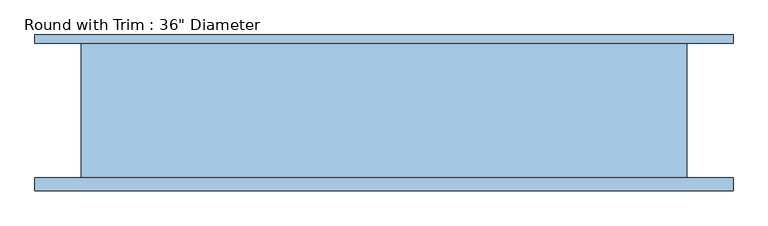
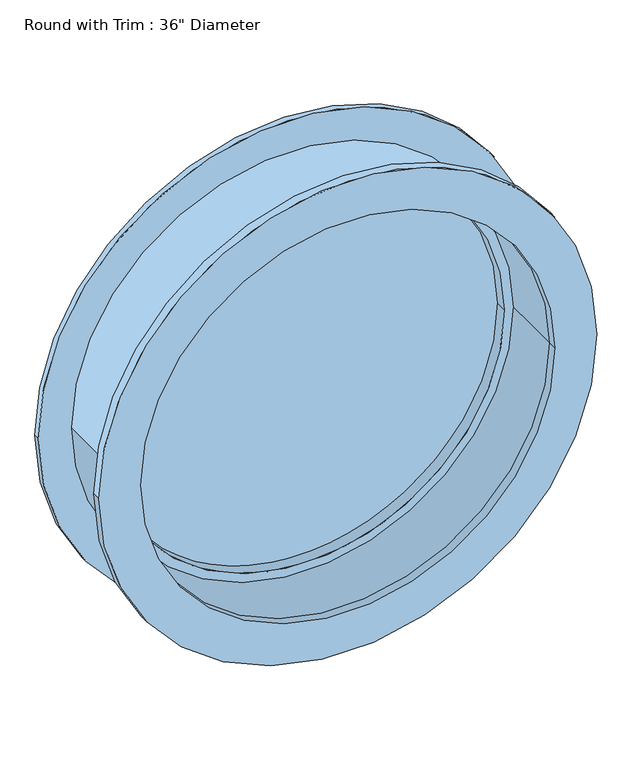
"""IFC4 building model written with IfcOpenShell, lengths in millimetres: window geometry."""

from ifc_helpers import new_model, si_unit, point, frame, frame_2d, origin, place, context, project, spatial, circle_curve, trimmed, segment, composite_curve, outline, extrude, source, transform, mapped, element, save


def window_736d8d37(model_context):
    return source(origin(), model_context, "Body", "SweptSolid", [
        extrude(outline(composite_curve([segment(trimmed(circle_curve(frame_2d((1219.2, 0.0)), 527.05), [point((1219.2, -527.05))], [point((1219.2, 527.05))], False, "CARTESIAN"), True, "CONTINUOUS"), segment(trimmed(circle_curve(frame_2d((1219.2, 0.0)), 527.05), [point((1219.2, 527.05))], [point((1219.2, -527.05))], False, "CARTESIAN"), True, "CONTINUOUS")], self_intersect=False), holes=[composite_curve([segment(trimmed(circle_curve(frame_2d((1219.2, 0.0)), 438.15), [point((1219.2, -438.15))], [point((1219.2, 438.15))], True, "CARTESIAN"), True, "CONTINUOUS"), segment(trimmed(circle_curve(frame_2d((1219.2, 0.0)), 438.15), [point((1219.2, 438.15))], [point((1219.2, -438.15))], True, "CARTESIAN"), True, "CONTINUOUS")], self_intersect=False)]), frame((0.0, -120.65, 0.0), z_axis=(0.0, 1.0, 0.0), x_axis=(0.0, 0.0, 1.0)), (0.0, 0.0, 1.0), 19.05),
        extrude(outline(composite_curve([segment(trimmed(circle_curve(frame_2d((1219.2, 0.0)), 527.05), [point((1219.2, -527.05))], [point((1219.2, 527.05))], False, "CARTESIAN"), True, "CONTINUOUS"), segment(trimmed(circle_curve(frame_2d((1219.2, 0.0)), 527.05), [point((1219.2, 527.05))], [point((1219.2, -527.05))], False, "CARTESIAN"), True, "CONTINUOUS")], self_intersect=False), holes=[composite_curve([segment(trimmed(circle_curve(frame_2d((1219.2, 0.0)), 438.15), [point((1219.2, -438.15))], [point((1219.2, 438.15))], True, "CARTESIAN"), True, "CONTINUOUS"), segment(trimmed(circle_curve(frame_2d((1219.2, 0.0)), 438.15), [point((1219.2, 438.15))], [point((1219.2, -438.15))], True, "CARTESIAN"), True, "CONTINUOUS")], self_intersect=False)]), frame((0.0, 101.6, 0.0), z_axis=(0.0, 1.0, 0.0), x_axis=(0.0, 0.0, 1.0)), (0.0, 0.0, 1.0), 12.7),
        extrude(outline(composite_curve([segment(trimmed(circle_curve(frame_2d((1219.2, 0.0)), 419.1), [point((1219.2, -419.1))], [point((1219.2, 419.1))], False, "CARTESIAN"), True, "CONTINUOUS"), segment(trimmed(circle_curve(frame_2d((1219.2, 0.0)), 419.1), [point((1219.2, 419.1))], [point((1219.2, -419.1))], False, "CARTESIAN"), True, "CONTINUOUS")], self_intersect=False)), frame((0.0, 57.15, 0.0), z_axis=(0.0, 1.0, 0.0), x_axis=(0.0, 0.0, 1.0)), (0.0, 0.0, 1.0), 12.7),
        extrude(outline(composite_curve([segment(trimmed(circle_curve(frame_2d((1219.2, 0.0)), 438.15), [point((1219.2, -438.15))], [point((1219.2, 438.15))], False, "CARTESIAN"), True, "CONTINUOUS"), segment(trimmed(circle_curve(frame_2d((1219.2, 0.0)), 438.15), [point((1219.2, 438.15))], [point((1219.2, -438.15))], False, "CARTESIAN"), True, "CONTINUOUS")], self_intersect=False), holes=[composite_curve([segment(trimmed(circle_curve(frame_2d((1219.2, 0.0)), 419.1), [point((1219.2, -419.1))], [point((1219.2, 419.1))], True, "CARTESIAN"), True, "CONTINUOUS"), segment(trimmed(circle_curve(frame_2d((1219.2, 0.0)), 419.1), [point((1219.2, 419.1))], [point((1219.2, -419.1))], True, "CARTESIAN"), True, "CONTINUOUS")], self_intersect=False)]), frame((0.0, 31.75, 0.0), z_axis=(0.0, 1.0, 0.0), x_axis=(0.0, 0.0, 1.0)), (0.0, 0.0, 1.0), 50.8),
        extrude(outline(composite_curve([segment(trimmed(circle_curve(frame_2d((1219.2, 0.0)), 457.2), [point((1219.2, -457.2))], [point((1219.2, 457.2))], False, "CARTESIAN"), True, "CONTINUOUS"), segment(trimmed(circle_curve(frame_2d((1219.2, 0.0)), 457.2), [point((1219.2, 457.2))], [point((1219.2, -457.2))], False, "CARTESIAN"), True, "CONTINUOUS")], self_intersect=False), holes=[composite_curve([segment(trimmed(circle_curve(frame_2d((1219.2, 0.0)), 438.15), [point((1219.2, -438.15))], [point((1219.2, 438.15))], True, "CARTESIAN"), True, "CONTINUOUS"), segment(trimmed(circle_curve(frame_2d((1219.2, 0.0)), 438.15), [point((1219.2, 438.15))], [point((1219.2, -438.15))], True, "CARTESIAN"), True, "CONTINUOUS")], self_intersect=False)]), frame((0.0, -101.6, 0.0), z_axis=(0.0, 1.0, 0.0), x_axis=(0.0, 0.0, 1.0)), (0.0, 0.0, 1.0), 203.2),
    ])


if __name__ == "__main__":
    model = new_model("IFC4")
    model_context = context("Model", 3, world=origin())
    ifc_project = project(units=[si_unit("LENGTHUNIT", "METRE", prefix="MILLI")], contexts=[model_context])
    site = spatial("IfcSite", under=ifc_project)
    building = spatial("IfcBuilding", under=site)
    placement = place(None, origin())
    window_shape = window_736d8d37(model_context)
    element("IfcWindow", 1, ObjectType="Round with Trim : 36\" Diameter", at=placement, inside=building, context=model_context, shape_type="MappedRepresentation", body=[
        mapped(window_shape, transform((0.0, 0.0, 0.0), x_axis=(1.0, 0.0, 0.0), y_axis=(0.0, 1.0, 0.0), z_axis=(0.0, 0.0, 1.0))),
    ])
    save(model, "model.ifc")

# Revit data of these elements
# Type "Round with Trim : 36\" Diameter"
#   Type Mark = "24"
#   Construction Type Id = "GSP4R"
#   Assembly Code = "B2020100"
#   Analytic Construction = "1/8 in Pilkington single glazing"
#   Visual Light Transmittance = 0.9
#   Solar Heat Gain Coefficient = 0.78
#   Heat Transfer Coefficient (U) = 0.6496 BTU/(h·ft²·°F)
#   Default Sill Height = 2' - 6"
#   Trim Projection - Ext. = 0' - 0 1/2"
#   Trim Projection - Int. = 0' - 0 3/4"
#   Trim Width - Exterior = 0' - 3 1/2"
#   Trim Width - Interior = 0' - 3 1/2"
#   Width = 3' - 0"
#   Define Thermal Properties by = 1
#   Glass Pane Material = Glass
#   Sash Material = Sash
#   Trim Exterior Material = Trim
#   Trim Interior Material = Trim
#   Wall Closure = (empty or 0)
# Element 1 (IfcWindow, "Round with Trim : 36\" Diameter")
#   Materials on its faces: "Trim", "Sash", "Glass"
# Materials
#   "Glass": class "Glass", colour RGB 0 128 192, transparency 0.75, Description = "Soda Lime Glass", Cost = 0
#   "Sash": class "Wood", colour RGB 224 178 126, transparency 0
#   "Trim": class "Wood", colour RGB 224 178 126, transparency 0
